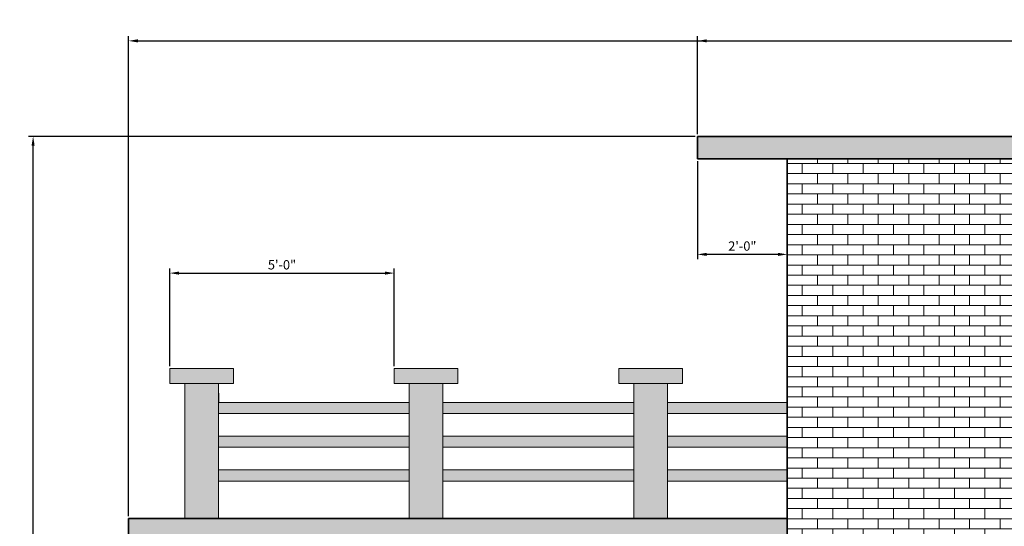
# Model space of a CAD drawing. Units: inches. Extents: x 4878 to 9282, y 5367 to 6617.
# Tile 2 of 14: x 4936 to 5199, y 5596 to 5731. Entities that reach past the tile are written whole.
import ezdxf

# ---------------------------------------------------------------- set-up
doc = ezdxf.new("R2010")
doc.units = ezdxf.units.IN
for name, color, linetype, lineweight in [('A-ANNO-DIMS', 2, 'Continuous', 18), ('A-ELEV', 7, 'Continuous', 35), ('A-ELEV-RAIL', 7, 'Continuous', 20), ('A-ELEV-RAIL-PATT', 7, 'Continuous', 13)]:
    doc.layers.add(name, color=color, linetype=linetype, lineweight=lineweight)
doc.layers.add('A-ELEV-CLAD-PATT', color=215, linetype='Continuous', lineweight=13, true_color=0xa953a0)
doc.layers.add('A-ELEV-TRIM-PATT', color=11, linetype='Continuous', lineweight=13, true_color=0xf27172)
doc.styles.get("Standard").update_dxf_attribs({"font": 'arial.ttf'})
doc.dimstyles.new('ISO-25', dxfattribs={"dimtxt": 2.5, "dimasz": 2.5, "dimexe": 1.25, "dimexo": 0.625, "dimtad": 1, "dimdec": 0, "dimlunit": 3, "dimtxsty": 'Standard', "dimcen": 2.5, "dimadec": 0, "dimazin": 0, "dimtfac": 1, "dimtdec": 0, "dimtmove": 0, "dimatfit": 3, "dimfxl": 1, "dimarcsym": 0})

# ---------------------------------------------------------------- blocks, each defined once
blk = doc.blocks.new('PARAPET-POST-CAPPED')
for p, q in [((0, 40), (0, 36)), ((0, 40), (17, 40)), ((17, 40), (17, 36)), ((0, 36), (17, 36)), ((4, 36), (4, 0)), ((13, 36), (13, 0))]:
    blk.add_line(p, q)
blk = doc.blocks.new('*D88')
at = {"layer": 'A-ANNO-DIMS', "color": 0, "lineweight": -2, "transparency": 16777216}
for p, q in [((4964.98, 5598.39), (4964.98, 5726.51)), ((4967.48, 5725.26), (5466.98, 5725.26)), ((5469.48, 5598.39), (5469.48, 5726.51))]:
    blk.add_line(p, q, dxfattribs=at)
at = {"layer": 'A-ANNO-DIMS', "color": 0, "transparency": 16777216}
for points in [[(4967.48, 5725.68), (4967.48, 5724.84), (4964.98, 5725.26)], [(5466.98, 5725.68), (5466.98, 5724.84), (5469.48, 5725.26)]]:
    blk.add_solid(points, dxfattribs=at)
at = {"layer": 'Defpoints', "color": 0, "transparency": 16777216}
for p in [(5469.48, 5725.26), (4964.98, 5597.76), (5469.48, 5597.76)]:
    blk.add_point(p, dxfattribs=at)
at = {"layer": 'A-ANNO-DIMS', "color": 0, "transparency": 16777216, "insert": (5217.23, 5727.18), "char_height": 2.5, "attachment_point": 5}
blk.add_mtext('42\'-0 1/2"', dxfattribs=at)
blk = doc.blocks.new('*D89')
at = {"layer": 'A-ANNO-DIMS', "color": 0, "lineweight": -2, "transparency": 16777216}
for p, q in [((5116.35, 5699.76), (4938.23, 5699.76)), ((4939.48, 5410.26), (4939.48, 5697.26)), ((5131.35, 5407.76), (4938.23, 5407.76))]:
    blk.add_line(p, q, dxfattribs=at)
at = {"layer": 'A-ANNO-DIMS', "color": 0, "transparency": 16777216}
for points in [[(4939.06, 5697.26), (4939.89, 5697.26), (4939.48, 5699.76)], [(4939.06, 5410.26), (4939.89, 5410.26), (4939.48, 5407.76)]]:
    blk.add_solid(points, dxfattribs=at)
at = {"layer": 'Defpoints', "color": 0, "transparency": 16777216}
for p in [(4939.48, 5699.76), (5116.98, 5699.76), (5131.98, 5407.76)]:
    blk.add_point(p, dxfattribs=at)
at = {"layer": 'A-ANNO-DIMS', "color": 0, "transparency": 16777216, "insert": (4937.6, 5553.76), "char_height": 2.5, "attachment_point": 5, "rotation": 90}
blk.add_mtext('24\'-4"', dxfattribs=at)
blk = doc.blocks.new('*D97')
at = {"layer": 'A-ANNO-DIMS', "color": 0, "lineweight": -2, "transparency": 16777216}
for p, q in [((4975.98, 5638.39), (4975.98, 5664.51)), ((5035.98, 5638.39), (5035.98, 5664.51)), ((4978.48, 5663.26), (5033.48, 5663.26))]:
    blk.add_line(p, q, dxfattribs=at)
at = {"layer": 'A-ANNO-DIMS', "color": 0, "transparency": 16777216}
for points in [[(4978.48, 5663.68), (4978.48, 5662.84), (4975.98, 5663.26)], [(5033.48, 5663.68), (5033.48, 5662.84), (5035.98, 5663.26)]]:
    blk.add_solid(points, dxfattribs=at)
at = {"layer": 'Defpoints', "color": 0, "transparency": 16777216}
for p in [(5035.98, 5663.26), (4975.98, 5637.76), (5035.98, 5637.76)]:
    blk.add_point(p, dxfattribs=at)
at = {"layer": 'A-ANNO-DIMS', "color": 0, "transparency": 16777216, "insert": (5005.98, 5665.16), "char_height": 2.5, "attachment_point": 5}
blk.add_mtext('5\'-0"', dxfattribs=at)
blk = doc.blocks.new('*D120')
at = {"layer": 'A-ANNO-DIMS', "color": 0, "lineweight": -2, "transparency": 16777216}
for p, q in [((5116.98, 5700.39), (5116.98, 5726.51)), ((5119.48, 5725.26), (5323.98, 5725.26)), ((5326.48, 5700.39), (5326.48, 5726.51))]:
    blk.add_line(p, q, dxfattribs=at)
at = {"layer": 'A-ANNO-DIMS', "color": 0, "transparency": 16777216}
for points in [[(5119.48, 5725.68), (5119.48, 5724.84), (5116.98, 5725.26)], [(5323.98, 5725.68), (5323.98, 5724.84), (5326.48, 5725.26)]]:
    blk.add_solid(points, dxfattribs=at)
at = {"layer": 'Defpoints', "color": 0, "transparency": 16777216}
for p in [(5326.48, 5725.26), (5116.98, 5699.76), (5326.48, 5699.76)]:
    blk.add_point(p, dxfattribs=at)
at = {"layer": 'A-ANNO-DIMS', "color": 0, "transparency": 16777216, "insert": (5221.73, 5727.18), "char_height": 2.5, "attachment_point": 5}
blk.add_mtext('17\'-5 1/2"', dxfattribs=at)
blk = doc.blocks.new('*D121')
at = {"layer": 'A-ANNO-DIMS', "color": 0, "lineweight": -2, "transparency": 16777216}
for p, q in [((5116.98, 5693.14), (5116.98, 5667.01)), ((5140.98, 5693.14), (5140.98, 5667.01)), ((5138.48, 5668.26), (5119.48, 5668.26))]:
    blk.add_line(p, q, dxfattribs=at)
at = {"layer": 'A-ANNO-DIMS', "color": 0, "transparency": 16777216}
for points in [[(5119.48, 5668.68), (5119.48, 5667.84), (5116.98, 5668.26)], [(5138.48, 5668.68), (5138.48, 5667.84), (5140.98, 5668.26)]]:
    blk.add_solid(points, dxfattribs=at)
at = {"layer": 'Defpoints', "color": 0, "transparency": 16777216}
for p in [(5116.98, 5693.76), (5140.98, 5693.76), (5116.98, 5668.26)]:
    blk.add_point(p, dxfattribs=at)
at = {"layer": 'A-ANNO-DIMS', "color": 0, "transparency": 16777216, "insert": (5128.98, 5670.16), "char_height": 2.5, "attachment_point": 5}
blk.add_mtext('2\'-0"', dxfattribs=at)

msp = doc.modelspace()

# ---------------------------------------------------------------- hatches: boundary and pattern name
at = {"layer": 'A-ELEV-CLAD-PATT'}
h = msp.add_hatch(dxfattribs=at)
h.set_pattern_fill('AR-BRSTD', color=256, scale=0.04)
h.set_pattern_definition([(0, (-2235.2307, 189.171), (0, 2.709672), []), (90, (-2235.2307, 189.171), (-4.064, 2.709672), [2.709672, -2.709672])])
h.paths.add_polyline_path([(5140.98, 5447.76), (5158.98, 5447.76), (5158.98, 5531.76), (5198.98, 5531.76), (5198.98, 5447.76), (5302.48, 5447.76), (5302.48, 5693.76), (5140.98, 5693.76)])
h.paths.add_polyline_path([(5225.95, 5537.76), (5279.95, 5537.76), (5279.95, 5531.76), (5273.95, 5531.76), (5273.95, 5495.76), (5231.95, 5495.76), (5231.95, 5531.76), (5225.95, 5531.76)], flags=16)
h.paths.add_polyline_path([(5234.95, 5528.76), (5270.95, 5528.76), (5270.95, 5498.76), (5234.95, 5498.76)], flags=0)
at = {"layer": 'A-ELEV-RAIL-PATT'}
h = msp.add_hatch(color=256, dxfattribs=at)
h.dxf.hatch_style = 1
h.paths.add_polyline_path([(5048.98, 5633.76), (5039.98, 5633.76), (5039.98, 5597.76), (5048.98, 5597.76)])
h.paths.add_polyline_path([(5108.98, 5633.76), (5099.98, 5633.76), (5099.98, 5597.76), (5108.98, 5597.76)])
h.paths.add_polyline_path([(4988.98, 5633.76), (4979.98, 5633.76), (4979.98, 5597.76), (4988.98, 5597.76)])
h.paths.add_polyline_path([(5334.48, 5633.76), (5325.48, 5633.76), (5325.48, 5597.76), (5334.48, 5597.76)])
h.paths.add_polyline_path([(5385.48, 5597.76), (5394.48, 5597.76), (5394.48, 5633.76), (5385.48, 5633.76)])
h.paths.add_polyline_path([(5445.48, 5597.76), (5454.48, 5597.76), (5454.48, 5633.76), (5445.48, 5633.76)])
h = msp.add_hatch(color=256, dxfattribs=at)
h.dxf.hatch_style = 1
h.paths.add_polyline_path([(5039.98, 5628.76), (4988.98, 5628.76), (4988.98, 5625.76), (5039.98, 5625.76)])
h.paths.add_polyline_path([(5099.98, 5628.76), (5048.98, 5628.76), (5048.98, 5625.76), (5099.98, 5625.76)])
h.paths.add_polyline_path([(5099.98, 5619.76), (5048.98, 5619.76), (5048.98, 5616.76), (5099.98, 5616.76)])
h.paths.add_polyline_path([(5099.98, 5610.76), (5048.98, 5610.76), (5048.98, 5607.76), (5099.98, 5607.76)])
h.paths.add_polyline_path([(5140.98, 5628.76), (5108.98, 5628.76), (5108.98, 5625.76), (5140.98, 5625.76)])
h.paths.add_polyline_path([(5140.98, 5619.76), (5108.98, 5619.76), (5108.98, 5616.76), (5140.98, 5616.76)])
h.paths.add_polyline_path([(5140.98, 5610.76), (5108.98, 5610.76), (5108.98, 5607.76), (5140.98, 5607.76)])
h.paths.add_polyline_path([(5325.48, 5610.76), (5302.48, 5610.76), (5302.48, 5607.76), (5325.48, 5607.76)])
h.paths.add_polyline_path([(5325.48, 5619.76), (5302.48, 5619.76), (5302.48, 5616.76), (5325.48, 5616.76)])
h.paths.add_polyline_path([(5325.48, 5628.76), (5302.48, 5628.76), (5302.48, 5625.76), (5325.48, 5625.76)])
h.paths.add_polyline_path([(5385.48, 5628.76), (5334.48, 5628.76), (5334.48, 5625.76), (5385.48, 5625.76)])
h.paths.add_polyline_path([(5385.48, 5619.76), (5334.48, 5619.76), (5334.48, 5616.76), (5385.48, 5616.76)])
h.paths.add_polyline_path([(5385.48, 5610.76), (5334.48, 5610.76), (5334.48, 5607.76), (5385.48, 5607.76)])
h.paths.add_polyline_path([(5445.48, 5628.76), (5394.48, 5628.76), (5394.48, 5625.76), (5445.48, 5625.76)])
h.paths.add_polyline_path([(5445.48, 5619.76), (5394.48, 5619.76), (5394.48, 5616.76), (5445.48, 5616.76)])
h.paths.add_polyline_path([(5445.48, 5610.76), (5394.48, 5610.76), (5394.48, 5607.76), (5445.48, 5607.76)])
h = msp.add_hatch(color=256, dxfattribs=at)
h.dxf.hatch_style = 1
h.paths.add_polyline_path([(5039.98, 5619.76), (4988.98, 5619.76), (4988.98, 5616.76), (5039.98, 5616.76)])
h.paths.add_polyline_path([(5039.98, 5610.76), (4988.98, 5610.76), (4988.98, 5607.76), (5039.98, 5607.76)])
at = {"layer": 'A-ELEV-TRIM-PATT'}
h = msp.add_hatch(color=256, dxfattribs=at)
h.dxf.hatch_style = 1
h.paths.add_polyline_path([(5140.98, 5591.76), (5140.98, 5597.76), (4964.98, 5597.76), (4964.98, 5591.76)])
h.paths.add_polyline_path([(5112.98, 5633.76), (5112.98, 5637.76), (5095.98, 5637.76), (5095.98, 5633.76)])
h.paths.add_polyline_path([(5035.98, 5637.76), (5035.98, 5633.76), (5052.98, 5633.76), (5052.98, 5637.76)])
h.paths.add_polyline_path([(4975.98, 5637.76), (4975.98, 5633.76), (4992.98, 5633.76), (4992.98, 5637.76)])
h.paths.add_polyline_path([(5116.98, 5699.76), (5116.98, 5693.76), (5326.48, 5693.76), (5326.48, 5699.76)])
h.paths.add_polyline_path([(5321.48, 5637.76), (5321.48, 5633.76), (5338.48, 5633.76), (5338.48, 5637.76)])
h.paths.add_polyline_path([(5381.48, 5637.76), (5381.48, 5633.76), (5398.48, 5633.76), (5398.48, 5637.76)])
h.paths.add_polyline_path([(5441.48, 5637.76), (5441.48, 5633.76), (5458.48, 5633.76), (5458.48, 5637.76)])
h.paths.add_polyline_path([(5469.48, 5591.76), (5469.48, 5597.76), (5302.48, 5597.76), (5302.48, 5591.76)])
h.paths.add_polyline_path([(5346.98, 5537.76), (5346.98, 5531.76), (5400.98, 5531.76), (5400.98, 5537.76)])
h.paths.add_polyline_path([(5279.95, 5531.76), (5279.95, 5537.76), (5225.95, 5537.76), (5225.95, 5531.76)])

# ---------------------------------------------------------------- linework, layer by layer
at = {"layer": 'A-ELEV'}
for p, q in [((5116.98, 5699.76), (5326.48, 5699.76)), ((5116.98, 5699.76), (5116.98, 5693.76)), ((5116.98, 5693.76), (5326.48, 5693.76)), ((5140.98, 5693.76), (5140.98, 5447.76)), ((4964.98, 5597.76), (5140.98, 5597.76)), ((4964.98, 5597.76), (4964.98, 5591.76))]:
    msp.add_line(p, q, dxfattribs=at)
at = {"layer": 'A-ELEV-RAIL'}
for p, q in [((4988.98, 5633.76), (4989.07, 5628.76)), ((4989.07, 5628.76), (5039.98, 5628.76)), ((5048.98, 5628.76), (5099.98, 5628.76)), ((5108.98, 5628.76), (5140.98, 5628.76)), ((4989.07, 5625.76), (5039.98, 5625.76)), ((5048.98, 5625.76), (5099.98, 5625.76)), ((5108.98, 5625.76), (5140.98, 5625.76)), ((4989.07, 5619.76), (5039.98, 5619.76)), ((5048.98, 5619.76), (5099.98, 5619.76)), ((5108.98, 5619.76), (5140.98, 5619.76)), ((4989.07, 5616.76), (5039.98, 5616.76)), ((5048.98, 5616.76), (5099.98, 5616.76)), ((5108.98, 5616.76), (5140.98, 5616.76)), ((4989.07, 5610.76), (5039.98, 5610.76)), ((5048.98, 5610.76), (5099.98, 5610.76)), ((5108.98, 5610.76), (5140.98, 5610.76)), ((4989.07, 5607.76), (5039.98, 5607.76)), ((5048.98, 5607.76), (5099.98, 5607.76)), ((5108.98, 5607.76), (5140.98, 5607.76))]:
    msp.add_line(p, q, dxfattribs=at)

# ---------------------------------------------------------------- block references
for p in [(4975.98, 5597.76), (5035.98, 5597.76), (5095.98, 5597.76)]:
    msp.add_blockref('PARAPET-POST-CAPPED', p, dxfattribs=at)

# ---------------------------------------------------------------- dimensions: what is measured, and where the dimension line sits
at = {"layer": 'A-ANNO-DIMS'}
for base, p1, p2, picture, middle in [((5469.48, 5725.26), (4964.98, 5597.76), (5469.48, 5597.76), '*D88', (5217.23, 5727.18)), ((5326.48, 5725.26), (5116.98, 5699.76), (5326.48, 5699.76), '*D120', (5221.73, 5727.18)), ((5035.98, 5663.26), (4975.98, 5637.76), (5035.98, 5637.76), '*D97', (5005.98, 5665.16))]:
    dim = msp.add_linear_dim(base=base, p1=p1, p2=p2, dimstyle='ISO-25', override={"dimdec": 1, "dimlfac": 1, "dimrnd": 0, "dimzin": 1, "dimdsep": 46, "dimlunit": 4, "dimfrac": 2}, dxfattribs=at)
    dim.commit()
    dim.dimension.update_dxf_attribs({"geometry": picture, "text_midpoint": middle})
for base, p1, p2, angle, picture, middle in [((4939.48, 5699.76), (5131.98, 5407.76), (5116.98, 5699.76), 90, '*D89', (4937.6, 5553.76)), ((5116.98, 5668.26), (5140.98, 5693.76), (5116.98, 5693.76), 180, '*D121', (5128.98, 5670.16))]:
    dim = msp.add_linear_dim(base=base, p1=p1, p2=p2, angle=angle, dimstyle='ISO-25', override={"dimdec": 1, "dimlfac": 1, "dimrnd": 0, "dimzin": 1, "dimdsep": 46, "dimlunit": 4, "dimfrac": 2}, dxfattribs=at)
    dim.commit()
    dim.dimension.update_dxf_attribs({"geometry": picture, "text_midpoint": middle})

doc.saveas('drawing.dxf')
